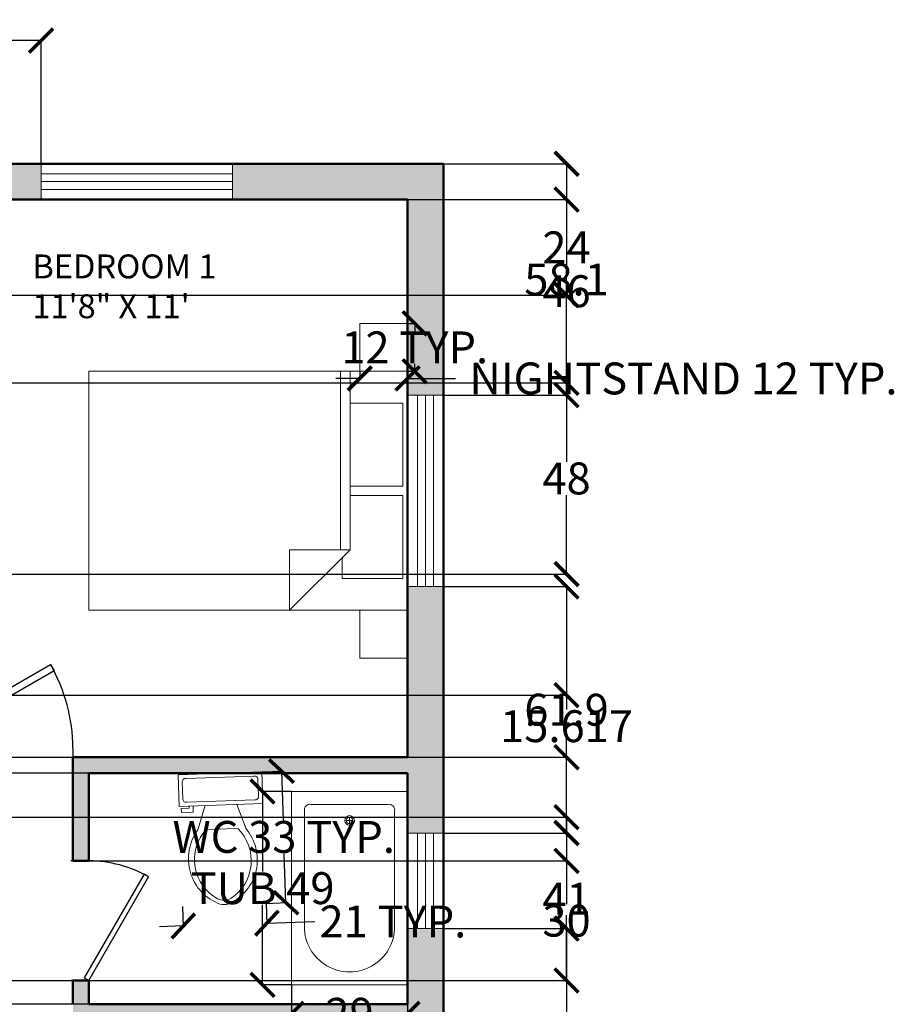
# Model space of a CAD drawing. Units: inches. Extents: x -30 to 744, y -375 to 57.
# Tile 8 of 8: x 525 to 744, y -190 to 57. Entities that reach past the tile are written whole.
import ezdxf

# ---------------------------------------------------------------- set-up
doc = ezdxf.new("R2010")
doc.units = ezdxf.units.IN
doc.header["$MEASUREMENT"] = 0
for name, color, linetype, lineweight in [('A-ANNO-DIMS', 2, 'Continuous', 18), ('A-AREA-IDEN', 7, 'Continuous', 25), ('A-DOOR', 3, 'Continuous', 25), ('A-FLOR-FIXT', 9, 'Continuous', 20), ('A-FURN', 8, 'Continuous', 18), ('A-GLAZ', 4, 'Continuous', 18), ('A-WALL', 7, 'Continuous', 50)]:
    doc.layers.add(name, color=color, linetype=linetype, lineweight=lineweight)
doc.layers.add('A-WALL-PATT', color=251, linetype='Continuous', lineweight=13, true_color=0x636466)
doc.styles.get("Standard").update_dxf_attribs({"font": 'arial.ttf'})
doc.dimstyles.get("Standard").update_dxf_attribs({"dimtxt": 8, "dimasz": 6, "dimexe": 0.18, "dimexo": 0.0625, "dimgap": 0.09, "dimtad": 0, "dimtih": 1, "dimtoh": 1, "dimdec": 0, "dimzin": 0, "dimdsep": 46, "dimlunit": 4, "dimtxsty": 'Standard', "dimblk": 'ARCHTICK', "dimcen": 0.09, "dimadec": 0, "dimazin": 0, "dimtfac": 1, "dimtdec": 0, "dimtofl": 0, "dimtmove": 0, "dimatfit": 1, "dimldrblk": 'ARCHTICK', "dimfxl": 1, "dimtolj": 1, "dimtzin": 0, "dimarcsym": 0})

# ---------------------------------------------------------------- blocks, each defined once
blk = doc.blocks.new('*U2')
for p, q in [((0, 0), (0, -6)), ((40, 0), (40, -6))]:
    blk.add_line(p, q)
blk.add_lwpolyline([(0, 0), (34.64, 20), (35.52, 18.48), (0.87, -1.52)], close=True)
blk.add_arc((0, 0), 40, 0, 30)
blk = doc.blocks.new('*U4')
for p, q in [((0, 0), (0, 6)), ((40, 0), (40, 6))]:
    blk.add_line(p, q)
blk.add_lwpolyline([(0, 0), (34.64, -20), (35.52, -18.48), (0.87, 1.52)], close=True)
blk.add_arc((0, 0), 40, 330, 0)
blk = doc.blocks.new('Bath Tub - 26 x 60 in.')
for p, q in [((8, -18), (10, -18)), ((9, -17), (9, -19))]:
    blk.add_line(p, q)
blk.add_lwpolyline([(0, -36), (0, 0), (60, 0), (60, -36)], close=True)
for points in [[(4, -30), (4, -6)], [(6, -4), (42, -4)], [(42, -32), (6, -32)]]:
    blk.add_lwpolyline(points)
for radius in [1.5, 1]:
    blk.add_circle((9, -18), radius)
for centre, radius, start, end in [((5.75, -5.75), 1.77, 81.8699, 188.1301), ((42, -18), 14, 270, 90), ((5.75, -30.25), 1.77, 171.8699, 278.1301)]:
    blk.add_arc(centre, radius, start, end)
blk = doc.blocks.new('Toilet - top')
for p, q in [((9.5, -6), (9.5, -2)), ((-10, -8.5), (-8, -8.5)), ((-10, -9.5), (-10, -8.5)), ((-7, -9.5), (-10, -9.5)), ((-8, -8.5), (-8, -8)), ((-7, -8), (-7, -9.5)), ((-4, -8), (-6, -14)), ((4, -8), (6, -14)), ((4, -14), (-4, -14))]:
    blk.add_line(p, q)
blk.add_lwpolyline([(10.5, -8), (10.5, 0), (-10.5, 0), (-10.5, -8)], close=True)
for points in [[(-9.5, -2), (-9.5, -6)], [(8.5, -1), (-8.5, -1)], [(-8.5, -7), (8.5, -7)]]:
    blk.add_lwpolyline(points)
for centre, radius, start, end in [((-8.62, -1.88), 0.884, 81.8699, 188.1301), ((8.62, -1.88), 0.884, 351.8699, 98.1301), ((-8.62, -6.12), 0.884, 171.8699, 278.1301), ((8.62, -6.12), 0.884, 261.8699, 8.1301), ((3.52, -21.58), 12.17, 141.4691, 247.9714), ((4.2, -21.82), 11.33, 136.3677, 238.9468), ((-3.52, -21.58), 12.17, 292.0284, 38.5307), ((-4.2, -21.82), 11.33, 301.053, 43.6321), ((0, -27.88), 4, 245.7318, 294.2682), ((0, -29), 4, 254.8605, 285.1395)]:
    blk.add_arc(centre, radius, start, end)
blk = doc.blocks.new('Bed - Queen')
for p, q in [((0, -80.00003), (0, 0)), ((0, 0), (59.99999, 0)), ((59.99999, 0), (59.99999, -80.00003)), ((7.99999, -1.2), (28.79998, -1.2)), ((7.99999, -14.4), (7.99999, -1.2)), ((28.79998, -1.2), (28.79998, -14.4)), ((31.19999, -1.2), (51.99999, -1.2)), ((31.19999, -14.4), (31.19999, -1.2)), ((51.99999, -1.2), (51.99999, -16.4)), ((0, -14.4), (44.8, -14.4)), ((59.99999, -29.6), (44.8, -14.4)), ((44.8, -14.4), (44.8, -29.6)), ((44.8, -16.8), (0, -16.8)), ((51.99999, -16.4), (46.79936, -16.4)), ((44.8, -29.6), (59.99999, -29.6)), ((59.99999, -80.00003), (0, -80.00003))]:
    blk.add_line(p, q)
blk = doc.blocks.new('WIN-48IN')
for p, q in [((0, 0), (0, 48)), ((0, 48), (9, 48)), ((2.5, 48), (2.5, 0)), ((4.5, 48), (4.5, 0)), ((6.5, 48), (6.5, 0)), ((9, 48), (9, 0)), ((9, 48), (9, 0)), ((9, 0), (0, 0))]:
    blk.add_line(p, q)
blk = doc.blocks.new('WIN-24IN')
for p, q in [((0, 0), (0, 9)), ((0, 9), (24, 9)), ((24, 0), (24, 9)), ((24, 6.5), (0, 6.5)), ((24, 4.5), (0, 4.5)), ((24, 2.5), (0, 2.5)), ((24, 0), (0, 0)), ((24, 0), (0, 0))]:
    blk.add_line(p, q)
blk = doc.blocks.new('NIGHTSTAND-12IN')
blk.add_lwpolyline([(0, 12), (0, 0), (12, 0), (12, 12)], close=True)
blk = doc.blocks.new('_ArchTick')
at = {"color": 0, "linetype": 'ByBlock', "const_width": 0.15}
blk.add_lwpolyline([(-0.5, -0.5), (0.5, 0.5)], dxfattribs=at)
blk = doc.blocks.new('*D30')
at = {"layer": 'A-ANNO-DIMS', "color": 0, "lineweight": -2, "transparency": 16777216}
for p, q in [((610.24, -31.46), (610.24, -33.38)), ((622.24, -31.46), (622.24, -33.38)), ((610.24, -33.2), (604.24, -33.2)), ((622.24, -33.2), (634.24, -33.2))]:
    blk.add_line(p, q, dxfattribs=at)
at = {"layer": 'Defpoints', "color": 0, "transparency": 16777216}
for p in [(610.24, -31.4), (622.24, -31.4), (622.24, -33.2)]:
    blk.add_point(p, dxfattribs=at)
at = {"layer": 'A-ANNO-DIMS', "color": 0, "lineweight": -2, "transparency": 16777216, "xscale": 6, "yscale": 6, "zscale": 6}
blk.add_blockref('_ArchTick', (610.24, -33.2), dxfattribs=at)
at = {"layer": 'A-ANNO-DIMS', "color": 0, "lineweight": -2, "transparency": 16777216, "xscale": 6, "yscale": 6, "zscale": 6, "rotation": 180}
blk.add_blockref('_ArchTick', (622.24, -33.2), dxfattribs=at)
at = {"layer": 'A-ANNO-DIMS', "color": 0, "transparency": 16777216, "insert": (691.48, -33.2), "char_height": 8, "attachment_point": 5}
blk.add_mtext('\\A1;NIGHTSTAND 12 TYP.', dxfattribs=at)
blk = doc.blocks.new('*D31')
at = {"layer": 'A-ANNO-DIMS', "color": 0, "lineweight": -2, "transparency": 16777216}
for p, q in [((622.3, -19.4), (624.22, -19.4)), ((624.04, -19.4), (624.04, -21.29)), ((624.04, -31.4), (624.04, -29.51)), ((622.3, -31.4), (624.22, -31.4))]:
    blk.add_line(p, q, dxfattribs=at)
at = {"layer": 'Defpoints', "color": 0, "transparency": 16777216}
for p in [(622.24, -19.4), (624.04, -19.4), (622.24, -31.4)]:
    blk.add_point(p, dxfattribs=at)
at = {"layer": 'A-ANNO-DIMS', "color": 0, "lineweight": -2, "transparency": 16777216, "xscale": 6, "yscale": 6, "zscale": 6}
for p, rotation in [((624.04, -19.4), 90), ((624.04, -31.4), 270)]:
    blk.add_blockref('_ArchTick', p, dxfattribs=dict(at, rotation=rotation))
at = {"layer": 'A-ANNO-DIMS', "color": 0, "transparency": 16777216, "insert": (624.04, -25.4), "char_height": 8, "attachment_point": 5}
blk.add_mtext('\\A1;12 TYP.', dxfattribs=at)
blk = doc.blocks.new('*D36')
at = {"layer": 'A-ANNO-DIMS', "color": 0, "lineweight": -2, "transparency": 16777216}
for p, q in [((593.05, -136.87), (585.66, -136.87)), ((585.84, -136.87), (585.84, -156.96)), ((585.84, -185.4), (585.84, -165.31)), ((593.05, -185.4), (585.66, -185.4))]:
    blk.add_line(p, q, dxfattribs=at)
at = {"layer": 'Defpoints', "color": 0, "transparency": 16777216}
for p in [(593.12, -136.87), (585.84, -185.4), (593.12, -185.4)]:
    blk.add_point(p, dxfattribs=at)
at = {"layer": 'A-ANNO-DIMS', "color": 0, "lineweight": -2, "transparency": 16777216, "xscale": 6, "yscale": 6, "zscale": 6}
for p, rotation in [((585.84, -136.87), 90), ((585.84, -185.4), 270)]:
    blk.add_blockref('_ArchTick', p, dxfattribs=dict(at, rotation=rotation))
at = {"layer": 'A-ANNO-DIMS', "color": 0, "transparency": 16777216, "insert": (585.84, -161.14), "char_height": 8, "attachment_point": 5}
blk.add_mtext('\\A1;TUB 49', dxfattribs=at)
blk = doc.blocks.new('*D37')
at = {"layer": 'A-ANNO-DIMS', "color": 0, "lineweight": -2, "transparency": 16777216}
for p, q in [((593.12, -185.47), (593.12, -192.86)), ((622.24, -185.47), (622.24, -192.86)), ((593.12, -192.68), (601.78, -192.68)), ((622.24, -192.68), (613.57, -192.68))]:
    blk.add_line(p, q, dxfattribs=at)
at = {"layer": 'Defpoints', "color": 0, "transparency": 16777216}
for p in [(593.12, -185.4), (622.24, -185.4), (622.24, -192.68)]:
    blk.add_point(p, dxfattribs=at)
at = {"layer": 'A-ANNO-DIMS', "color": 0, "lineweight": -2, "transparency": 16777216, "xscale": 6, "yscale": 6, "zscale": 6, "rotation": 180}
blk.add_blockref('_ArchTick', (593.12, -192.68), dxfattribs=at)
at = {"layer": 'A-ANNO-DIMS', "color": 0, "lineweight": -2, "transparency": 16777216, "xscale": 6, "yscale": 6, "zscale": 6}
blk.add_blockref('_ArchTick', (622.24, -192.68), dxfattribs=at)
at = {"layer": 'A-ANNO-DIMS', "color": 0, "transparency": 16777216, "insert": (607.68, -192.68), "char_height": 8, "attachment_point": 5}
blk.add_mtext('\\A1;29', dxfattribs=at)
blk = doc.blocks.new('*D40')
at = {"layer": 'A-ANNO-DIMS', "color": 0, "lineweight": -2, "transparency": 16777216}
for p, q in [((585.69, -131.93), (590.77, -131.76)), ((590.59, -131.76), (591.01, -144.05)), ((591.72, -164.79), (591.3, -152.51)), ((586.83, -164.96), (591.9, -164.78))]:
    blk.add_line(p, q, dxfattribs=at)
at = {"layer": 'Defpoints', "color": 0, "transparency": 16777216}
for p in [(585.63, -131.93), (590.59, -131.76), (586.77, -164.96)]:
    blk.add_point(p, dxfattribs=at)
at = {"layer": 'A-ANNO-DIMS', "color": 0, "lineweight": -2, "transparency": 16777216, "xscale": 6, "yscale": 6, "zscale": 6}
for p, rotation in [((590.59, -131.76), 91.97634423977817), ((591.72, -164.79), 271.9763442397782)]:
    blk.add_blockref('_ArchTick', p, dxfattribs=dict(at, rotation=rotation))
at = {"layer": 'A-ANNO-DIMS', "color": 0, "transparency": 16777216, "insert": (591.16, -148.28), "char_height": 8, "attachment_point": 5}
blk.add_mtext('\\A1;WC 33 TYP.', dxfattribs=at)
blk = doc.blocks.new('*D41')
at = {"layer": 'A-ANNO-DIMS', "color": 0, "lineweight": -2, "transparency": 16777216}
for p, q in [((586.77, -165.02), (586.95, -170.1)), ((565.79, -165.75), (565.96, -170.82)), ((586.94, -169.92), (598.93, -169.5)), ((565.95, -170.64), (559.96, -170.85))]:
    blk.add_line(p, q, dxfattribs=at)
at = {"layer": 'Defpoints', "color": 0, "transparency": 16777216}
for p in [(586.77, -164.96), (565.78, -165.69), (586.94, -169.92)]:
    blk.add_point(p, dxfattribs=at)
at = {"layer": 'A-ANNO-DIMS', "color": 0, "lineweight": -2, "transparency": 16777216, "xscale": 6, "yscale": 6, "zscale": 6}
for p, rotation in [((565.95, -170.64), 1.976344239778278), ((586.94, -169.92), 181.9763442397782)]:
    blk.add_blockref('_ArchTick', p, dxfattribs=dict(at, rotation=rotation))
at = {"layer": 'A-ANNO-DIMS', "color": 0, "transparency": 16777216, "insert": (618.56, -169.5), "char_height": 8, "attachment_point": 5}
blk.add_mtext('\\A1;21 TYP.', dxfattribs=at)
blk = doc.blocks.new('*D63')
at = {"layer": 'A-ANNO-DIMS', "color": 0, "lineweight": -2, "transparency": 16777216}
for p, q in [((542.17, -132.3), (-16.61, -132.3)), ((-16.43, -132.3), (-16.43, -157.12)), ((-16.43, -190.3), (-16.43, -165.47)), ((542.17, -190.3), (-16.61, -190.3))]:
    blk.add_line(p, q, dxfattribs=at)
at = {"layer": 'Defpoints', "color": 0, "transparency": 16777216}
for p in [(-16.43, -132.3), (542.24, -132.3), (542.24, -190.3)]:
    blk.add_point(p, dxfattribs=at)
at = {"layer": 'A-ANNO-DIMS', "color": 0, "lineweight": -2, "transparency": 16777216, "xscale": 6, "yscale": 6, "zscale": 6}
for p, rotation in [((-16.43, -132.3), 90), ((-16.43, -190.3), 270)]:
    blk.add_blockref('_ArchTick', p, dxfattribs=dict(at, rotation=rotation))
at = {"layer": 'A-ANNO-DIMS', "color": 0, "transparency": 16777216, "insert": (-16.43, -161.3), "char_height": 8, "attachment_point": 5}
blk.add_mtext('\\A1;58', dxfattribs=at)
blk = doc.blocks.new('*D72')
at = {"layer": 'A-ANNO-DIMS', "color": 0, "lineweight": -2, "transparency": 16777216}
for p, q in [((453.51, 20.77), (453.51, 51.78)), ((453.51, 51.6), (478.34, 51.6)), ((530.27, 51.6), (505.45, 51.6)), ((530.27, 20.77), (530.27, 51.78))]:
    blk.add_line(p, q, dxfattribs=at)
at = {"layer": 'Defpoints', "color": 0, "transparency": 16777216}
for p in [(530.27, 51.6), (453.51, 20.7), (530.27, 20.7)]:
    blk.add_point(p, dxfattribs=at)
at = {"layer": 'A-ANNO-DIMS', "color": 0, "lineweight": -2, "transparency": 16777216, "xscale": 6, "yscale": 6, "zscale": 6, "rotation": 180}
blk.add_blockref('_ArchTick', (453.51, 51.6), dxfattribs=at)
at = {"layer": 'A-ANNO-DIMS', "color": 0, "lineweight": -2, "transparency": 16777216, "xscale": 6, "yscale": 6, "zscale": 6}
blk.add_blockref('_ArchTick', (530.27, 51.6), dxfattribs=at)
at = {"layer": 'A-ANNO-DIMS', "color": 0, "transparency": 16777216, "insert": (491.89, 51.6), "char_height": 8, "attachment_point": 5}
blk.add_mtext('\\A1;76.76', dxfattribs=at)
blk = doc.blocks.new('*D75')
at = {"layer": 'A-ANNO-DIMS', "color": 0, "lineweight": -2, "transparency": 16777216}
for p, q in [((40.3, 11.7), (662.32, 11.7)), ((662.14, 11.7), (662.14, -7.12)), ((662.14, -34.3), (662.14, -15.47)), ((40.3, -34.3), (662.32, -34.3))]:
    blk.add_line(p, q, dxfattribs=at)
at = {"layer": 'Defpoints', "color": 0, "transparency": 16777216}
for p in [(40.24, 11.7), (662.14, 11.7), (40.24, -34.3)]:
    blk.add_point(p, dxfattribs=at)
at = {"layer": 'A-ANNO-DIMS', "color": 0, "lineweight": -2, "transparency": 16777216, "xscale": 6, "yscale": 6, "zscale": 6}
for p, rotation in [((662.14, 11.7), 90), ((662.14, -34.3), 270)]:
    blk.add_blockref('_ArchTick', p, dxfattribs=dict(at, rotation=rotation))
at = {"layer": 'A-ANNO-DIMS', "color": 0, "transparency": 16777216, "insert": (662.14, -11.3), "char_height": 8, "attachment_point": 5}
blk.add_mtext('\\A1;46', dxfattribs=at)
blk = doc.blocks.new('*D76')
at = {"layer": 'A-ANNO-DIMS', "color": 0, "lineweight": -2, "transparency": 16777216}
for p, q in [((631.3, 20.7), (662.32, 20.7)), ((662.14, 20.7), (662.14, -4.17)), ((662.14, -37.4), (662.14, -12.52)), ((631.3, -37.4), (662.32, -37.4))]:
    blk.add_line(p, q, dxfattribs=at)
at = {"layer": 'Defpoints', "color": 0, "transparency": 16777216}
for p in [(631.24, 20.7), (662.14, 20.7), (631.24, -37.4)]:
    blk.add_point(p, dxfattribs=at)
at = {"layer": 'A-ANNO-DIMS', "color": 0, "lineweight": -2, "transparency": 16777216, "xscale": 6, "yscale": 6, "zscale": 6}
for p, rotation in [((662.14, 20.7), 90), ((662.14, -37.4), 270)]:
    blk.add_blockref('_ArchTick', p, dxfattribs=dict(at, rotation=rotation))
at = {"layer": 'A-ANNO-DIMS', "color": 0, "transparency": 16777216, "insert": (662.14, -8.35), "char_height": 8, "attachment_point": 5}
blk.add_mtext('\\A1;58.1', dxfattribs=at)
blk = doc.blocks.new('*D77')
at = {"layer": 'A-ANNO-DIMS', "color": 0, "lineweight": -2, "transparency": 16777216}
for p, q in [((631.3, -85.4), (662.32, -85.4)), ((662.14, -85.4), (662.14, -112.17)), ((662.14, -147.3), (662.14, -120.52)), ((631.3, -147.3), (662.32, -147.3))]:
    blk.add_line(p, q, dxfattribs=at)
at = {"layer": 'Defpoints', "color": 0, "transparency": 16777216}
for p in [(631.24, -85.4), (662.14, -85.4), (631.24, -147.3)]:
    blk.add_point(p, dxfattribs=at)
at = {"layer": 'A-ANNO-DIMS', "color": 0, "lineweight": -2, "transparency": 16777216, "xscale": 6, "yscale": 6, "zscale": 6}
for p, rotation in [((662.14, -85.4), 90), ((662.14, -147.3), 270)]:
    blk.add_blockref('_ArchTick', p, dxfattribs=dict(at, rotation=rotation))
at = {"layer": 'A-ANNO-DIMS', "color": 0, "transparency": 16777216, "insert": (662.14, -116.35), "char_height": 8, "attachment_point": 5}
blk.add_mtext('\\A1;61.9', dxfattribs=at)
blk = doc.blocks.new('*D78')
at = {"layer": 'A-ANNO-DIMS', "color": 0, "lineweight": -2, "transparency": 16777216}
for p, q in [((631.3, -171.3), (662.32, -171.3)), ((662.14, -171.3), (662.14, -200.21)), ((662.14, -237.46), (662.14, -208.55)), ((631.3, -237.46), (662.32, -237.46))]:
    blk.add_line(p, q, dxfattribs=at)
at = {"layer": 'Defpoints', "color": 0, "transparency": 16777216}
for p in [(631.24, -171.3), (662.14, -171.3), (631.24, -237.46)]:
    blk.add_point(p, dxfattribs=at)
at = {"layer": 'A-ANNO-DIMS', "color": 0, "lineweight": -2, "transparency": 16777216, "xscale": 6, "yscale": 6, "zscale": 6}
for p, rotation in [((662.14, -171.3), 90), ((662.14, -237.46), 270)]:
    blk.add_blockref('_ArchTick', p, dxfattribs=dict(at, rotation=rotation))
at = {"layer": 'A-ANNO-DIMS', "color": 0, "transparency": 16777216, "insert": (662.14, -204.38), "char_height": 8, "attachment_point": 5}
blk.add_mtext('\\A1;66.17', dxfattribs=at)
blk = doc.blocks.new('*D79')
at = {"layer": 'A-ANNO-DIMS', "color": 0, "lineweight": -2, "transparency": 16777216}
for p, q in [((542.3, -154.3), (662.32, -154.3)), ((662.14, -154.3), (662.14, -165.12)), ((662.14, -184.3), (662.14, -173.47)), ((542.3, -184.3), (662.32, -184.3))]:
    blk.add_line(p, q, dxfattribs=at)
at = {"layer": 'Defpoints', "color": 0, "transparency": 16777216}
for p in [(542.24, -154.3), (662.14, -154.3), (542.24, -184.3)]:
    blk.add_point(p, dxfattribs=at)
at = {"layer": 'A-ANNO-DIMS', "color": 0, "lineweight": -2, "transparency": 16777216, "xscale": 6, "yscale": 6, "zscale": 6}
for p, rotation in [((662.14, -154.3), 90), ((662.14, -184.3), 270)]:
    blk.add_blockref('_ArchTick', p, dxfattribs=dict(at, rotation=rotation))
at = {"layer": 'A-ANNO-DIMS', "color": 0, "transparency": 16777216, "insert": (662.14, -169.3), "char_height": 8, "attachment_point": 5}
blk.add_mtext('\\A1;30', dxfattribs=at)
blk = doc.blocks.new('*D80')
at = {"layer": 'A-ANNO-DIMS', "color": 0, "lineweight": -2, "transparency": 16777216}
for p, q in [((120.38, -143.3), (662.32, -143.3)), ((662.14, -143.3), (662.14, -159.69)), ((662.14, -184.3), (662.14, -167.9)), ((120.38, -184.3), (662.32, -184.3))]:
    blk.add_line(p, q, dxfattribs=at)
at = {"layer": 'Defpoints', "color": 0, "transparency": 16777216}
for p in [(120.31, -143.3), (662.14, -143.3), (120.31, -184.3)]:
    blk.add_point(p, dxfattribs=at)
at = {"layer": 'A-ANNO-DIMS', "color": 0, "lineweight": -2, "transparency": 16777216, "xscale": 6, "yscale": 6, "zscale": 6}
for p, rotation in [((662.14, -143.3), 90), ((662.14, -184.3), 270)]:
    blk.add_blockref('_ArchTick', p, dxfattribs=dict(at, rotation=rotation))
at = {"layer": 'A-ANNO-DIMS', "color": 0, "transparency": 16777216, "insert": (662.14, -163.8), "char_height": 8, "attachment_point": 5}
blk.add_mtext('\\A1;41', dxfattribs=at)
blk = doc.blocks.new('*D82')
at = {"layer": 'A-ANNO-DIMS', "color": 0, "lineweight": -2, "transparency": 16777216}
for p, q in [((366.3, -34.3), (662.32, -34.3)), ((662.14, -34.3), (662.14, -54.12)), ((662.14, -82.3), (662.14, -62.47)), ((366.3, -82.3), (662.32, -82.3))]:
    blk.add_line(p, q, dxfattribs=at)
at = {"layer": 'Defpoints', "color": 0, "transparency": 16777216}
for p in [(366.24, -34.3), (366.24, -82.3), (662.14, -82.3)]:
    blk.add_point(p, dxfattribs=at)
at = {"layer": 'A-ANNO-DIMS', "color": 0, "lineweight": -2, "transparency": 16777216, "xscale": 6, "yscale": 6, "zscale": 6}
for p, rotation in [((662.14, -34.3), 90), ((662.14, -82.3), 270)]:
    blk.add_blockref('_ArchTick', p, dxfattribs=dict(at, rotation=rotation))
at = {"layer": 'A-ANNO-DIMS', "color": 0, "transparency": 16777216, "insert": (662.14, -58.3), "char_height": 8, "attachment_point": 5}
blk.add_mtext('\\A1;48', dxfattribs=at)
blk = doc.blocks.new('*D84')
at = {"layer": 'A-ANNO-DIMS', "color": 0, "lineweight": -2, "transparency": 16777216}
for p, q in [((366.3, 11.7), (662.32, 11.7)), ((662.14, 11.7), (662.14, 3.81)), ((662.14, -12.3), (662.14, -4.4)), ((366.3, -12.3), (662.32, -12.3))]:
    blk.add_line(p, q, dxfattribs=at)
at = {"layer": 'Defpoints', "color": 0, "transparency": 16777216}
for p in [(366.24, 11.7), (366.24, -12.3), (662.14, -12.3)]:
    blk.add_point(p, dxfattribs=at)
at = {"layer": 'A-ANNO-DIMS', "color": 0, "lineweight": -2, "transparency": 16777216, "xscale": 6, "yscale": 6, "zscale": 6}
for p, rotation in [((662.14, 11.7), 90), ((662.14, -12.3), 270)]:
    blk.add_blockref('_ArchTick', p, dxfattribs=dict(at, rotation=rotation))
at = {"layer": 'A-ANNO-DIMS', "color": 0, "transparency": 16777216, "insert": (662.14, -0.3), "char_height": 8, "attachment_point": 5}
blk.add_mtext('\\A1;24', dxfattribs=at)
blk = doc.blocks.new('*D90')
at = {"layer": 'A-ANNO-DIMS', "color": 0, "lineweight": -2, "transparency": 16777216}
for p, q in [((208.3, -112.68), (662.32, -112.68)), ((662.14, -112.68), (662.14, -116.31)), ((662.14, -128.3), (662.14, -124.66)), ((208.3, -128.3), (662.32, -128.3))]:
    blk.add_line(p, q, dxfattribs=at)
at = {"layer": 'Defpoints', "color": 0, "transparency": 16777216}
for p in [(208.24, -112.68), (208.24, -128.3), (662.14, -128.3)]:
    blk.add_point(p, dxfattribs=at)
at = {"layer": 'A-ANNO-DIMS', "color": 0, "lineweight": -2, "transparency": 16777216, "xscale": 6, "yscale": 6, "zscale": 6}
for p, rotation in [((662.14, -112.68), 90), ((662.14, -128.3), 270)]:
    blk.add_blockref('_ArchTick', p, dxfattribs=dict(at, rotation=rotation))
at = {"layer": 'A-ANNO-DIMS', "color": 0, "transparency": 16777216, "insert": (662.14, -120.49), "char_height": 8, "attachment_point": 5}
blk.add_mtext('\\A1;15.617', dxfattribs=at)

msp = doc.modelspace()

# ---------------------------------------------------------------- hatches: boundary and pattern name
at = {"layer": 'A-WALL-PATT'}
h = msp.add_hatch(color=256, dxfattribs=at)
h.dxf.hatch_style = 1
h.paths.add_polyline_path([(40.2356, 11.7031), (204.2356, 11.7031), (204.2356, -24.2969), (208.2356, -24.2969), (208.2356, 11.7031), (233.4275, 11.7031), (233.4275, 20.7031), (31.2356, 20.7031), (31.2356, -34.2969), (40.2356, -34.2969)])
h.paths.add_polyline_path([(40.2356, -82.2969), (31.2356, -82.2969), (31.2356, -132.2969), (40.2356, -132.2969), (51.0767, -132.2969), (111.3137, -132.2969), (111.3137, -143.2969), (120.3137, -143.2969), (120.3137, -132.2969), (156.2356, -132.2969), (156.2356, -128.2969), (113.6001, -128.2969), (113.6001, -128.3034), (53.6001, -128.3034), (40.2356, -128.2969)])
h.paths.add_polyline_path([(302.4681, 20.7031), (257.4275, 20.7031), (257.4275, 11.7031), (286.2356, 11.7031), (286.2356, -60.2969), (208.2356, -60.2969), (208.2356, -54.2969), (204.2356, -54.2969), (204.2356, -64.2969), (208.2356, -64.2969), (286.2356, -64.2969), (286.2356, -128.2969), (264.8954, -128.2969), (208.2356, -128.2969), (204.2356, -128.2969), (198.2356, -128.2969), (198.2356, -132.2969), (290.2356, -132.2969), (290.2356, -128.2969), (290.2356, 11.7031), (302.4681, 11.7031)])
h.paths.add_polyline_path([(405.515, 20.7031), (350.4681, 20.7031), (350.4681, 11.7031), (362.2356, 11.7031), (362.2356, -34.2969), (366.2356, -34.2969), (366.2356, 11.7031), (405.515, 11.7031)])
h.paths.add_polyline_path([(530.2713, 20.7031), (453.515, 20.7031), (453.515, 11.7031), (486.2356, 11.7031), (486.2356, -128.2969), (448.2356, -128.2969), (448.2356, -132.2969), (486.2356, -132.2969), (490.2356, -132.2969), (496.2356, -132.2969), (496.2356, -128.2969), (490.2356, -128.2969), (490.2356, 11.7031), (530.2713, 11.7031)])
h.paths.add_polyline_path([(631.2356, 20.7031), (578.2713, 20.7031), (578.2713, 11.7031), (622.2356, 11.7031), (622.2356, -37.4001), (631.2356, -37.4001)])
h.paths.add_polyline_path([(631.2356, -85.4001), (622.2356, -85.4001), (622.2356, -91.4001), (622.2356, -103.4001), (622.2356, -128.2969), (538.2356, -128.2969), (538.2356, -132.2969), (538.2356, -154.2969), (542.2356, -154.2969), (542.2356, -132.2969), (575.1375, -132.2969), (585.6313, -131.9348), (585.6438, -132.2969), (622.2356, -132.2969), (622.2356, -147.2969), (631.2356, -147.2969)])
h.paths.add_polyline_path([(631.2356, -171.2969), (622.2356, -171.2969), (622.2356, -185.4028), (622.2356, -186.2969), (622.2356, -190.2969), (542.2356, -190.2969), (542.2356, -184.2969), (538.2356, -184.2969), (538.2356, -190.2969), (538.2356, -194.2969), (622.2356, -194.2969), (622.2356, -237.4632), (631.2356, -237.4632)])
h.paths.add_polyline_path([(631.2356, -285.4632), (622.2356, -285.4632), (622.2356, -330.2969), (490.2356, -330.2969), (490.2356, -194.2969), (494.2356, -194.2969), (495.2356, -194.2969), (495.2356, -190.2969), (494.2356, -190.2969), (490.2356, -190.2969), (486.2356, -190.2969), (366.2356, -190.2969), (366.2356, -194.2969), (486.2356, -194.2969), (486.2356, -330.2969), (426.2356, -330.2969), (426.2356, -339.2969), (631.2356, -339.2969)])
h.paths.add_polyline_path([(378.2356, -330.2969), (318.2356, -330.2969), (318.2356, -194.2969), (324.2356, -194.2969), (324.2356, -190.2969), (318.2356, -190.2969), (314.2356, -190.2969), (314.2356, -194.2969), (314.2356, -330.2969), (278.2356, -330.2969), (278.2356, -339.2969), (378.2356, -339.2969)])
h.paths.add_polyline_path([(190.2356, -330.2969), (40.2356, -330.2969), (40.2356, -318.2969), (31.2356, -318.2969), (31.2356, -330.2969), (31.2356, -339.2969), (190.2356, -339.2969)])
h.paths.add_polyline_path([(230.2356, -330.2969), (194.2356, -330.2969), (194.2356, -194.2969), (194.2356, -190.2969), (190.2356, -190.2969), (184.2356, -190.2969), (184.2356, -194.2969), (190.2356, -194.2969), (190.2356, -339.2969), (230.2356, -339.2969)])
h.paths.add_polyline_path([(142.2356, -190.2969), (120.3137, -190.2969), (120.3137, -184.2969), (116.3137, -184.2969), (111.3137, -184.2969), (111.3137, -190.2969), (40.2356, -190.2969), (31.2356, -190.2969), (31.2356, -194.2969), (31.2356, -206.2969), (40.2356, -206.2969), (40.2356, -194.2969), (142.2356, -194.2969)])

# ---------------------------------------------------------------- linework, layer by layer
at = {"layer": 'A-WALL'}
for p, q in [((490.2356, 11.7031), (622.2356, 11.7031)), ((622.2356, 11.7031), (622.2356, -128.2969)), ((538.2356, -128.2969), (538.2356, -132.2969)), ((538.2356, -128.2969), (622.2356, -128.2969)), ((538.2356, -128.2969), (622.2356, -128.2969)), ((538.2356, -154.2969), (538.2356, -132.2969)), ((542.2356, -154.2969), (542.2356, -132.2969)), ((622.2356, -132.2969), (542.2356, -132.2969)), ((622.2356, -132.2969), (622.2356, -186.2969)), ((538.2356, -154.2969), (542.2356, -154.2969)), ((538.2356, -190.2969), (538.2356, -184.2969)), ((538.2356, -184.2969), (542.2356, -184.2969)), ((542.2356, -184.2969), (542.2356, -190.2969)), ((622.2356, -186.2969), (622.2356, -190.2969)), ((622.2356, -190.2969), (542.2356, -190.2969))]:
    msp.add_line(p, q, dxfattribs=at)
msp.add_lwpolyline([(31.2356, -132.2969), (31.2356, 20.7031), (631.2356, 20.7031), (631.2356, -339.2969), (190.2356, -339.2969)], dxfattribs=at)

# ---------------------------------------------------------------- block references
at = {"layer": 'A-DOOR', "xscale": 1.05, "yscale": 1.05, "zscale": 1.05}
msp.add_blockref('*U2', (496.2356, -125.9969), dxfattribs=at)
at = {"layer": 'A-DOOR', "xscale": 0.75, "yscale": 0.75, "zscale": 0.75, "rotation": 90}
msp.add_blockref('*U4', (542.2356, -184.2969), dxfattribs=at)
at = {"layer": 'A-FLOR-FIXT', "rotation": 1.976344239778263}
msp.add_blockref('Toilet - top', (575.1375, -132.2969), dxfattribs=at)
at = {"layer": 'A-FLOR-FIXT', "xscale": 0.8088859012127309, "yscale": 0.8088859012127309, "zscale": 0.8088859012127309, "rotation": 270}
msp.add_blockref('Bath Tub - 26 x 60 in.', (622.2356, -136.8696), dxfattribs=at)
at = {"layer": 'A-FURN'}
for p in [(610.236, -31.4), (610.236, -103.4)]:
    msp.add_blockref('NIGHTSTAND-12IN', p, dxfattribs=at)
at = {"layer": 'A-FURN', "rotation": 270}
msp.add_blockref('Bed - Queen', (622.2356, -31.4001), dxfattribs=at)
at = {"layer": 'A-GLAZ'}
for name, p, rotation in [('WIN-48IN', (530.2714, 20.7027), 270.0000000000003), ('WIN-24IN', (622.2354, -147.2973), 270)]:
    msp.add_blockref(name, p, dxfattribs=dict(at, rotation=rotation))
msp.add_blockref('WIN-48IN', (622.236, -85.4), dxfattribs=at)

# ---------------------------------------------------------------- texts
at = {"layer": 'A-AREA-IDEN', "insert": (528.0726, -2.0764), "char_height": 6, "attachment_point": 1}
msp.add_mtext_dynamic_manual_height_columns('BEDROOM 1\\P11\'8" X 11\'', width=82.162914, gutter_width=1, heights=[0], dxfattribs=at)

# ---------------------------------------------------------------- dimensions: what is measured, and where the dimension line sits
at = {"layer": 'A-ANNO-DIMS'}
for base, p1, p2, override, picture, middle in [((530.2713, 51.6031), (453.515, 20.7031), (530.2713, 20.7031), {"dimdec": 2, "dimlfac": 1, "dimrnd": 0, "dimzin": 0, "dimdsep": 46, "dimlunit": 2}, '*D72', (491.8931, 51.6031)), ((622.2356, -192.6828), (593.1157, -185.4028), (622.2356, -185.4028), {"dimdec": 0, "dimlfac": 1, "dimrnd": 0, "dimzin": 0, "dimdsep": 46, "dimlunit": 2}, '*D37', (607.6756, -192.6828))]:
    dim = msp.add_linear_dim(base=base, p1=p1, p2=p2, dimstyle='Standard', override=override, dxfattribs=at)
    dim.commit()
    dim.dimension.update_dxf_attribs({"geometry": picture, "text_midpoint": middle})
for base, p1, p2, override, picture, middle in [((662.1356, 20.7031), (631.2356, -37.4001), (631.2356, 20.7031), {"dimdec": 1, "dimlfac": 1, "dimrnd": 0, "dimzin": 0, "dimdsep": 46, "dimlunit": 2}, '*D76', (662.1356, -8.3485)), ((662.1356, 11.7031), (40.2356, -34.2969), (40.2356, 11.7031), {"dimdec": 0, "dimlfac": 1, "dimrnd": 0, "dimzin": 0, "dimdsep": 46, "dimlunit": 2}, '*D75', (662.1356, -11.2969)), ((662.1356, -12.2969), (366.2356, 11.7031), (366.2356, -12.2969), {"dimdec": 0, "dimlfac": 1, "dimrnd": 0, "dimzin": 0, "dimdsep": 46, "dimlunit": 2}, '*D84', (662.1356, -0.2969)), ((662.1356, -82.2969), (366.2356, -34.2969), (366.2356, -82.2969), {"dimdec": 0, "dimlfac": 1, "dimrnd": 0, "dimzin": 0, "dimdsep": 46, "dimlunit": 2}, '*D82', (662.1356, -58.2969)), ((662.1356, -85.4001), (631.2356, -147.2969), (631.2356, -85.4001), {"dimdec": 1, "dimlfac": 1, "dimrnd": 0, "dimzin": 0, "dimdsep": 46, "dimlunit": 2}, '*D77', (662.1356, -116.3485)), ((662.1356, -128.2969), (208.2356, -112.6796), (208.2356, -128.2969), {"dimdec": 3, "dimlfac": 1, "dimrnd": 0, "dimzin": 0, "dimdsep": 46, "dimlunit": 2}, '*D90', (662.1356, -120.4882)), ((-16.4253, -132.2969), (542.2356, -190.2969), (542.2356, -132.2969), {"dimdec": 0, "dimlfac": 1, "dimrnd": 0, "dimzin": 0, "dimdsep": 46, "dimlunit": 2}, '*D63', (-16.4253, -161.2969)), ((662.1356, -143.2969), (120.3137, -184.2969), (120.3137, -143.2969), {"dimdec": 0, "dimlfac": 1, "dimrnd": 0, "dimzin": 0, "dimdsep": 46, "dimlunit": 2}, '*D80', (662.1356, -163.7969)), ((662.1356, -154.2969), (542.2356, -184.2969), (542.2356, -154.2969), {"dimdec": 0, "dimlfac": 1, "dimrnd": 0, "dimzin": 0, "dimdsep": 46, "dimlunit": 2}, '*D79', (662.1356, -169.2969)), ((662.1356, -171.2969), (631.2356, -237.4632), (631.2356, -171.2969), {"dimdec": 2, "dimlfac": 1, "dimrnd": 0, "dimzin": 0, "dimdsep": 46, "dimlunit": 2}, '*D78', (662.1356, -204.38))]:
    dim = msp.add_linear_dim(base=base, p1=p1, p2=p2, angle=90, dimstyle='Standard', override=override, dxfattribs=at)
    dim.commit()
    dim.dimension.update_dxf_attribs({"geometry": picture, "text_midpoint": middle})
dim = msp.add_linear_dim(base=(622.2356, -33.2001), p1=(610.2356, -31.4001), p2=(622.2356, -31.4001), text='NIGHTSTAND <> TYP.', dimstyle='Standard', override={"dimdec": 0, "dimlfac": 1, "dimrnd": 0, "dimzin": 0, "dimdsep": 46, "dimlunit": 2}, dxfattribs=at)
dim.commit()
dim.dimension.update_dxf_attribs({"geometry": '*D30', "text_midpoint": (691.477, -33.2001)})
for base, p1, p2, angle, text, picture, middle in [((624.0356, -19.4001), (622.2356, -31.4001), (622.2356, -19.4001), 90, '<> TYP.', '*D31', (624.0356, -25.4001)), ((590.5853, -131.7638), (586.771, -164.9613), (585.6313, -131.9348), 91.976344, 'WC <> TYP.', '*D40', (591.1551, -148.2771)), ((585.8357, -185.4028), (593.1157, -136.8696), (593.1157, -185.4028), 270, 'TUB <>', '*D36', (585.8357, -161.1362)), ((586.9419, -169.9153), (565.7834, -165.6856), (586.771, -164.9613), 1.976344, '<> TYP.', '*D41', (618.5636, -169.5015))]:
    dim = msp.add_linear_dim(base=base, p1=p1, p2=p2, angle=angle, text=text, dimstyle='Standard', override={"dimdec": 0, "dimlfac": 1, "dimrnd": 0, "dimzin": 0, "dimdsep": 46, "dimlunit": 2}, dxfattribs=at)
    dim.commit()
    dim.dimension.update_dxf_attribs({"geometry": picture, "text_midpoint": middle})

doc.saveas('drawing.dxf')
